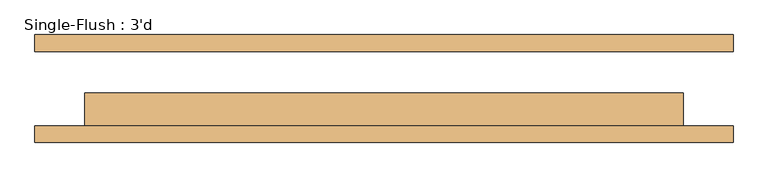
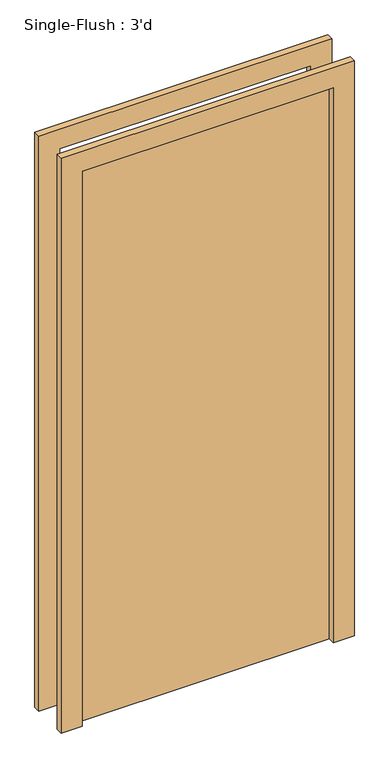
"""IFC4 building model written with IfcOpenShell, lengths in millimetres: door geometry, Single-Flush : 3'd."""

from ifc_helpers import new_model, si_unit, frame, origin, origin_with_axes, place, context, project, spatial, polyline, outline, extrude, source, transform, mapped, element, save


def single_flush_3_d_305aa2a5(model_context):
    return source(origin(), model_context, "Body", "SweptSolid", [
        extrude(outline(polyline([(2209.8, -533.4), (0.0, -533.4), (0.0, -457.2), (2133.6, -457.2), (2133.6, 457.2), (0.0, 457.2), (0.0, 533.4), (2209.8, 533.4), (2209.8, -533.4)])), frame((0.0, -82.55, 0.0), z_axis=(0.0, 1.0, 0.0), x_axis=(0.0, 0.0, 1.0)), (0.0, 0.0, 1.0), 25.4),
        extrude(outline(polyline([(2209.8, 533.4), (2209.8, -533.4), (0.0, -533.4), (0.0, -457.2), (2133.6, -457.2), (2133.6, 457.2), (0.0, 457.2), (0.0, 533.4), (2209.8, 533.4)])), frame((0.0, 57.15, 0.0), z_axis=(0.0, 1.0, 0.0), x_axis=(0.0, 0.0, 1.0)), (0.0, 0.0, 1.0), 25.4),
        extrude(outline(polyline([(457.2, -6.35), (457.2, -57.15), (-457.2, -57.15), (-457.2, -6.35), (457.2, -6.35)])), origin_with_axes(), (0.0, 0.0, 1.0), 2133.6),
    ])


if __name__ == "__main__":
    model = new_model("IFC4")
    model_context = context("Model", 3, world=origin())
    ifc_project = project(units=[si_unit("LENGTHUNIT", "METRE", prefix="MILLI")], contexts=[model_context])
    site = spatial("IfcSite", under=ifc_project)
    building = spatial("IfcBuilding", under=site)
    placement = place(None, origin())
    single_flush_3_d_shape = single_flush_3_d_305aa2a5(model_context)
    element("IfcDoor", 1, ObjectType="Single-Flush : 3'd", at=placement, inside=building, context=model_context, shape_type="MappedRepresentation", body=[
        mapped(single_flush_3_d_shape, transform((0.0, 0.0, 0.0), x_axis=(1.0, 0.0, 0.0), y_axis=(0.0, 1.0, 0.0), z_axis=(0.0, 0.0, 1.0))),
    ])
    save(model, "model.ifc")

# Revit data of these elements
# Type "Single-Flush : 3'd"
#   Type Mark = "13"
#   Construction Type Id = "MDOOR"
#   Assembly Code = "C1020"
#   Analytic Construction = "Metal"
#   Thickness = 0' - 2"
#   Heat Transfer Coefficient (U) = 0.651978 BTU/(h·ft²·°F)
#   Height = 7' - 0"
#   Trim Projection Ext = 0' - 1"
#   Trim Projection Int = 0' - 1"
#   Trim Width = 0' - 3"
#   Width = 3' - 0"
#   Define Thermal Properties by = 1
#   Door Material = Door - Panel
#   Frame Material = Door - Frame
#   Visual Light Transmittance = 0
#   Solar Heat Gain Coefficient = 0
#   Function = (empty or 0)
#   Wall Closure = (empty or 0)
# Element 1 (IfcDoor, "Single-Flush : 3'd")
#   Materials on its faces: "Door - Frame", "Door - Panel"
# Materials
#   "Door - Panel": class "Wood", colour RGB 210 159 95, transparency 0, Cost = 0
#   "Door - Frame": colour RGB 118 70 51, transparency 0, Cost = 0
